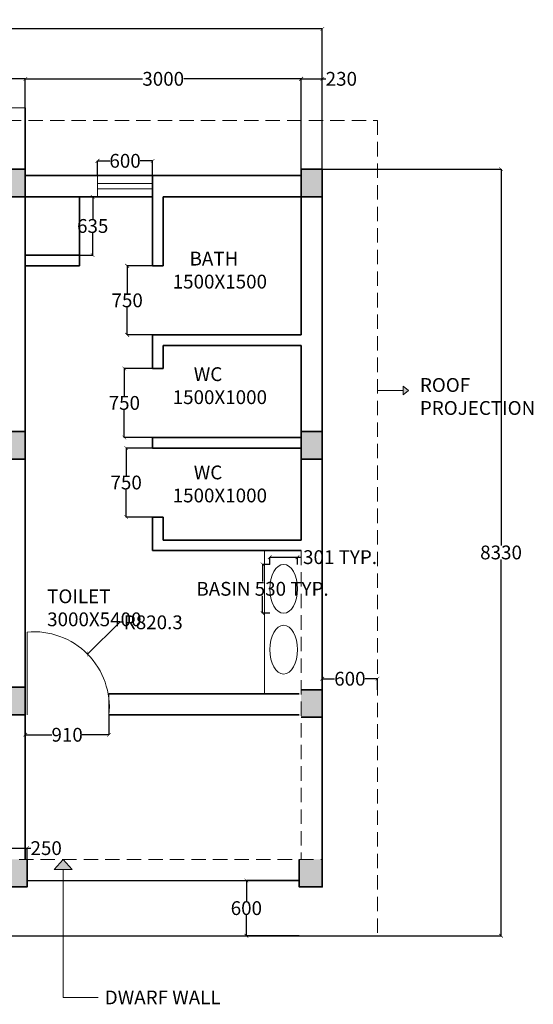
# Model space of a CAD drawing. Units: millimetres. Extents: x 32888 to 53184, y 27889 to 39696.
# Tile 6 of 6: x 47598 to 53184, y 28996 to 39696. Entities that reach past the tile are written whole.
import ezdxf

# ---------------------------------------------------------------- set-up
doc = ezdxf.new("R2010")
doc.units = ezdxf.units.MM
doc.header["$LTSCALE"] = 50
doc.header["$MEASUREMENT"] = 0
doc.linetypes.add('HIDDEN2', pattern=[0.1875, 0.125, -0.0625])
for name, color, linetype, lineweight in [('A-ANNO-DIMS', 2, 'Continuous', 18), ('A-ANNO-SYMB', 7, 'Continuous', 18), ('A-ANNO-SYMB-PATT', 18, 'Continuous', 13), ('A-ANNO-TEXT', 7, 'Continuous', 18), ('A-AREA-IDEN', 7, 'Continuous', 18), ('A-COLS', 1, 'Continuous', 35), ('A-COLS-PATT', 18, 'Continuous', 18), ('A-DOOR', 4, 'Continuous', 18), ('A-FLOR-FIXT', 9, 'Continuous', 18), ('A-GLAZ', 4, 'Continuous', 18), ('A-ROOF-OVHD', 8, 'HIDDEN2', 18), ('A-WALL', 7, 'Continuous', 35), ('A-WALL-HIDN', 7, 'HIDDEN2', 18), ('A-WALL-LOW', 7, 'Continuous', 25)]:
    doc.layers.add(name, color=color, linetype=linetype, lineweight=lineweight)
doc.styles.get("Standard").update_dxf_attribs({"font": 'arial.ttf'})
doc.dimstyles.get("Standard").update_dxf_attribs({"dimtxt": 150, "dimasz": 40, "dimexe": 0.18, "dimexo": 0.0625, "dimgap": 0.09, "dimtad": 0, "dimtih": 1, "dimtoh": 1, "dimdec": 0, "dimzin": 0, "dimdsep": 46, "dimtxsty": 'Standard', "dimblk": 'ARCHTICK', "dimcen": 0, "dimadec": 0, "dimazin": 0, "dimtfac": 1, "dimtdec": 0, "dimtofl": 0, "dimtmove": 0, "dimatfit": 3, "dimldrblk": 'ARCHTICK', "dimfxl": 1, "dimtolj": 1, "dimtzin": 0, "dimarcsym": 1})

# ---------------------------------------------------------------- blocks, each defined once
blk = doc.blocks.new('_ArchTick')
at = {"color": 0, "linetype": 'ByBlock', "const_width": 0.15}
blk.add_lwpolyline([(-0.5, -0.5), (0.5, 0.5)], dxfattribs=at)
blk = doc.blocks.new('*D8')
at = {"layer": 'A-ANNO-DIMS', "color": 0, "lineweight": -2, "ltscale": 50, "transparency": 16777216}
for p, q in [((47429, 30571), (47429, 30693)), ((47429, 30693), (47679, 30693)), ((47679, 30571), (47679, 30693)), ((47679, 30693), (47719, 30693))]:
    blk.add_line(p, q, dxfattribs=at)
at = {"layer": 'Defpoints', "color": 0, "ltscale": 50, "transparency": 16777216}
for p in [(47679, 30693), (47429, 30571), (47679, 30571)]:
    blk.add_point(p, dxfattribs=at)
at = {"layer": 'A-ANNO-DIMS', "color": 0, "lineweight": -2, "ltscale": 50, "transparency": 16777216, "xscale": 40, "yscale": 40, "zscale": 40, "rotation": 180}
blk.add_blockref('_ArchTick', (47429, 30693), dxfattribs=at)
at = {"layer": 'A-ANNO-DIMS', "color": 0, "lineweight": -2, "ltscale": 50, "transparency": 16777216, "xscale": 40, "yscale": 40, "zscale": 40}
blk.add_blockref('_ArchTick', (47679, 30693), dxfattribs=at)
at = {"layer": 'A-ANNO-DIMS', "color": 0, "ltscale": 50, "transparency": 16777216, "insert": (47886, 30693), "char_height": 150, "attachment_point": 5}
blk.add_mtext('\\A1;250', dxfattribs=at)
blk = doc.blocks.new('*D10')
at = {"layer": 'A-ANNO-DIMS', "color": 0, "lineweight": -2, "ltscale": 50, "transparency": 16777216}
for p, q in [((50639, 30341), (50063, 30341)), ((50063, 30341), (50063, 30118)), ((50063, 29741), (50063, 29964)), ((50639, 29741), (50063, 29741))]:
    blk.add_line(p, q, dxfattribs=at)
at = {"layer": 'Defpoints', "color": 0, "ltscale": 50, "transparency": 16777216}
for p in [(50639, 30341), (50063, 29741), (50639, 29741)]:
    blk.add_point(p, dxfattribs=at)
at = {"layer": 'A-ANNO-DIMS', "color": 0, "lineweight": -2, "ltscale": 50, "transparency": 16777216, "xscale": 40, "yscale": 40, "zscale": 40}
for p, rotation in [((50063, 30341), 90), ((50063, 29741), 270)]:
    blk.add_blockref('_ArchTick', p, dxfattribs=dict(at, rotation=rotation))
at = {"layer": 'A-ANNO-DIMS', "color": 0, "ltscale": 50, "transparency": 16777216, "insert": (50063, 30041), "char_height": 150, "attachment_point": 5}
blk.add_mtext('\\A1;600', dxfattribs=at)
blk = doc.blocks.new('*D11')
at = {"layer": 'A-ANNO-DIMS', "color": 0, "lineweight": -2, "ltscale": 50, "transparency": 16777216}
for p, q in [((50889, 32415), (50889, 32534)), ((50889, 32534), (51023, 32534)), ((51489, 32534), (51355, 32534)), ((51489, 32415), (51489, 32534))]:
    blk.add_line(p, q, dxfattribs=at)
at = {"layer": 'Defpoints', "color": 0, "ltscale": 50, "transparency": 16777216}
for p in [(51489, 32534), (50889, 32414), (51489, 32414)]:
    blk.add_point(p, dxfattribs=at)
at = {"layer": 'A-ANNO-DIMS', "color": 0, "lineweight": -2, "ltscale": 50, "transparency": 16777216, "xscale": 40, "yscale": 40, "zscale": 40, "rotation": 180}
blk.add_blockref('_ArchTick', (50889, 32534), dxfattribs=at)
at = {"layer": 'A-ANNO-DIMS', "color": 0, "lineweight": -2, "ltscale": 50, "transparency": 16777216, "xscale": 40, "yscale": 40, "zscale": 40}
blk.add_blockref('_ArchTick', (51489, 32534), dxfattribs=at)
at = {"layer": 'A-ANNO-DIMS', "color": 0, "ltscale": 50, "transparency": 16777216, "insert": (51189, 32534), "char_height": 150, "attachment_point": 5}
blk.add_mtext('\\A1;600', dxfattribs=at)
blk = doc.blocks.new('*D27')
at = {"layer": 'A-ANNO-DIMS', "color": 0, "lineweight": -2, "ltscale": 50, "transparency": 16777216}
for p, q in [((49044, 35041), (48756, 35041)), ((48756, 35041), (48756, 34743)), ((48756, 34291), (48756, 34589)), ((49044, 34291), (48756, 34291))]:
    blk.add_line(p, q, dxfattribs=at)
at = {"layer": 'Defpoints', "color": 0, "ltscale": 50, "transparency": 16777216}
for p in [(49044, 35041), (48756, 34291), (49044, 34291)]:
    blk.add_point(p, dxfattribs=at)
at = {"layer": 'A-ANNO-DIMS', "color": 0, "lineweight": -2, "ltscale": 50, "transparency": 16777216, "xscale": 40, "yscale": 40, "zscale": 40}
for p, rotation in [((48756, 35041), 90), ((48756, 34291), 270)]:
    blk.add_blockref('_ArchTick', p, dxfattribs=dict(at, rotation=rotation))
at = {"layer": 'A-ANNO-DIMS', "color": 0, "ltscale": 50, "transparency": 16777216, "insert": (48756, 34666), "char_height": 150, "attachment_point": 5}
blk.add_mtext('\\A1;750', dxfattribs=at)
blk = doc.blocks.new('*D28')
at = {"layer": 'A-ANNO-DIMS', "color": 0, "lineweight": -2, "ltscale": 50, "transparency": 16777216}
for p, q in [((49044, 35906), (48736, 35906)), ((48736, 35906), (48736, 35608)), ((48736, 35156), (48736, 35454)), ((49044, 35156), (48736, 35156))]:
    blk.add_line(p, q, dxfattribs=at)
at = {"layer": 'Defpoints', "color": 0, "ltscale": 50, "transparency": 16777216}
for p in [(49044, 35906), (48736, 35156), (49044, 35156)]:
    blk.add_point(p, dxfattribs=at)
at = {"layer": 'A-ANNO-DIMS', "color": 0, "lineweight": -2, "ltscale": 50, "transparency": 16777216, "xscale": 40, "yscale": 40, "zscale": 40}
for p, rotation in [((48736, 35906), 90), ((48736, 35156), 270)]:
    blk.add_blockref('_ArchTick', p, dxfattribs=dict(at, rotation=rotation))
at = {"layer": 'A-ANNO-DIMS', "color": 0, "ltscale": 50, "transparency": 16777216, "insert": (48736, 35531), "char_height": 150, "attachment_point": 5}
blk.add_mtext('\\A1;750', dxfattribs=at)
blk = doc.blocks.new('*D29')
at = {"layer": 'A-ANNO-DIMS', "color": 0, "lineweight": -2, "ltscale": 50, "transparency": 16777216}
for p, q in [((49044, 37021), (48767, 37021)), ((48767, 37021), (48767, 36723)), ((48767, 36271), (48767, 36569)), ((49044, 36271), (48767, 36271))]:
    blk.add_line(p, q, dxfattribs=at)
at = {"layer": 'Defpoints', "color": 0, "ltscale": 50, "transparency": 16777216}
for p in [(48767, 37021), (49044, 37021), (49044, 36271)]:
    blk.add_point(p, dxfattribs=at)
at = {"layer": 'A-ANNO-DIMS', "color": 0, "lineweight": -2, "ltscale": 50, "transparency": 16777216, "xscale": 40, "yscale": 40, "zscale": 40}
for p, rotation in [((48767, 37021), 90), ((48767, 36271), 270)]:
    blk.add_blockref('_ArchTick', p, dxfattribs=dict(at, rotation=rotation))
at = {"layer": 'A-ANNO-DIMS', "color": 0, "ltscale": 50, "transparency": 16777216, "insert": (48767, 36646), "char_height": 150, "attachment_point": 5}
blk.add_mtext('\\A1;750', dxfattribs=at)
blk = doc.blocks.new('*D30')
at = {"layer": 'A-ANNO-DIMS', "color": 0, "lineweight": -2, "ltscale": 50, "transparency": 16777216}
for p, q in [((48249, 37771), (48392, 37771)), ((48392, 37771), (48392, 37530)), ((48392, 37136), (48392, 37377)), ((48249, 37136), (48392, 37136))]:
    blk.add_line(p, q, dxfattribs=at)
at = {"layer": 'Defpoints', "color": 0, "ltscale": 50, "transparency": 16777216}
for p in [(48249, 37771), (48392, 37771), (48249, 37136)]:
    blk.add_point(p, dxfattribs=at)
at = {"layer": 'A-ANNO-DIMS', "color": 0, "lineweight": -2, "ltscale": 50, "transparency": 16777216, "xscale": 40, "yscale": 40, "zscale": 40}
for p, rotation in [((48392, 37771), 90), ((48392, 37136), 270)]:
    blk.add_blockref('_ArchTick', p, dxfattribs=dict(at, rotation=rotation))
at = {"layer": 'A-ANNO-DIMS', "color": 0, "ltscale": 50, "transparency": 16777216, "insert": (48392, 37454), "char_height": 150, "attachment_point": 5}
blk.add_mtext('\\A1;635', dxfattribs=at)
blk = doc.blocks.new('*D31')
at = {"layer": 'A-ANNO-DIMS', "color": 0, "lineweight": -2, "ltscale": 50, "transparency": 16777216}
for p, q in [((48444, 38001), (48444, 38162)), ((48444, 38162), (48578, 38162)), ((49044, 38162), (48910, 38162)), ((49044, 38001), (49044, 38162))]:
    blk.add_line(p, q, dxfattribs=at)
at = {"layer": 'Defpoints', "color": 0, "ltscale": 50, "transparency": 16777216}
for p in [(49044, 38162), (48444, 38001), (49044, 38001)]:
    blk.add_point(p, dxfattribs=at)
at = {"layer": 'A-ANNO-DIMS', "color": 0, "lineweight": -2, "ltscale": 50, "transparency": 16777216, "xscale": 40, "yscale": 40, "zscale": 40, "rotation": 180}
blk.add_blockref('_ArchTick', (48444, 38162), dxfattribs=at)
at = {"layer": 'A-ANNO-DIMS', "color": 0, "lineweight": -2, "ltscale": 50, "transparency": 16777216, "xscale": 40, "yscale": 40, "zscale": 40}
blk.add_blockref('_ArchTick', (49044, 38162), dxfattribs=at)
at = {"layer": 'A-ANNO-DIMS', "color": 0, "ltscale": 50, "transparency": 16777216, "insert": (48744, 38162), "char_height": 150, "attachment_point": 5}
blk.add_mtext('\\A1;600', dxfattribs=at)
blk = doc.blocks.new('*D48')
at = {"layer": 'A-ANNO-DIMS', "color": 0, "lineweight": -2, "ltscale": 50, "transparency": 16777216}
for p, q in [((50659, 38071), (50659, 39053)), ((50659, 39053), (50889, 39053)), ((50889, 38071), (50889, 39053)), ((50889, 39053), (50929, 39053))]:
    blk.add_line(p, q, dxfattribs=at)
at = {"layer": 'Defpoints', "color": 0, "ltscale": 50, "transparency": 16777216}
for p in [(50889, 39053), (50659, 38071), (50889, 38071)]:
    blk.add_point(p, dxfattribs=at)
at = {"layer": 'A-ANNO-DIMS', "color": 0, "lineweight": -2, "ltscale": 50, "transparency": 16777216, "xscale": 40, "yscale": 40, "zscale": 40, "rotation": 180}
blk.add_blockref('_ArchTick', (50659, 39053), dxfattribs=at)
at = {"layer": 'A-ANNO-DIMS', "color": 0, "lineweight": -2, "ltscale": 50, "transparency": 16777216, "xscale": 40, "yscale": 40, "zscale": 40}
blk.add_blockref('_ArchTick', (50889, 39053), dxfattribs=at)
at = {"layer": 'A-ANNO-DIMS', "color": 0, "ltscale": 50, "transparency": 16777216, "insert": (51096, 39053), "char_height": 150, "attachment_point": 5}
blk.add_mtext('\\A1;230', dxfattribs=at)
blk = doc.blocks.new('*D49')
at = {"layer": 'A-ANNO-DIMS', "color": 0, "lineweight": -2, "ltscale": 50, "transparency": 16777216}
for p, q in [((47659, 38001), (47659, 39053)), ((47659, 39053), (48935, 39053)), ((50659, 39053), (49383, 39053)), ((50659, 38001), (50659, 39053))]:
    blk.add_line(p, q, dxfattribs=at)
at = {"layer": 'Defpoints', "color": 0, "ltscale": 50, "transparency": 16777216}
for p in [(47659, 39053), (47659, 38001), (50659, 38001)]:
    blk.add_point(p, dxfattribs=at)
at = {"layer": 'A-ANNO-DIMS', "color": 0, "lineweight": -2, "ltscale": 50, "transparency": 16777216, "xscale": 40, "yscale": 40, "zscale": 40, "rotation": 180}
blk.add_blockref('_ArchTick', (47659, 39053), dxfattribs=at)
at = {"layer": 'A-ANNO-DIMS', "color": 0, "lineweight": -2, "ltscale": 50, "transparency": 16777216, "xscale": 40, "yscale": 40, "zscale": 40}
blk.add_blockref('_ArchTick', (50659, 39053), dxfattribs=at)
at = {"layer": 'A-ANNO-DIMS', "color": 0, "ltscale": 50, "transparency": 16777216, "insert": (49159, 39053), "char_height": 150, "attachment_point": 5}
blk.add_mtext('\\A1;3000', dxfattribs=at)
blk = doc.blocks.new('*D50')
at = {"layer": 'A-ANNO-DIMS', "color": 0, "lineweight": -2, "ltscale": 50, "transparency": 16777216}
for p, q in [((47429, 39053), (47389, 39053)), ((47429, 38071), (47429, 39053)), ((47659, 39053), (47429, 39053)), ((47659, 38071), (47659, 39053))]:
    blk.add_line(p, q, dxfattribs=at)
at = {"layer": 'Defpoints', "color": 0, "ltscale": 50, "transparency": 16777216}
for p in [(47429, 39053), (47429, 38071), (47659, 38071)]:
    blk.add_point(p, dxfattribs=at)
at = {"layer": 'A-ANNO-DIMS', "color": 0, "lineweight": -2, "ltscale": 50, "transparency": 16777216, "xscale": 40, "yscale": 40, "zscale": 40}
for p, rotation in [((47429, 39053), 179.9999999999982), ((47659, 39053), 359.9999999999982)]:
    blk.add_blockref('_ArchTick', p, dxfattribs=dict(at, rotation=rotation))
at = {"layer": 'A-ANNO-DIMS', "color": 0, "ltscale": 50, "transparency": 16777216, "insert": (47222, 39053), "char_height": 150, "attachment_point": 5}
blk.add_mtext('\\A1;230', dxfattribs=at)
blk = doc.blocks.new('*D56')
at = {"layer": 'A-ANNO-DIMS', "color": 0, "lineweight": -2, "ltscale": 50, "transparency": 16777216}
for p, q in [((47659, 32141), (47659, 31925)), ((48569, 32141), (48569, 31925)), ((47659, 31925), (47948, 31925)), ((48569, 31925), (48279, 31925))]:
    blk.add_line(p, q, dxfattribs=at)
at = {"layer": 'Defpoints', "color": 0, "ltscale": 50, "transparency": 16777216}
for p in [(47659, 32141), (48569, 32141), (47659, 31925)]:
    blk.add_point(p, dxfattribs=at)
at = {"layer": 'A-ANNO-DIMS', "color": 0, "lineweight": -2, "ltscale": 50, "transparency": 16777216, "xscale": 40, "yscale": 40, "zscale": 40, "rotation": 180}
blk.add_blockref('_ArchTick', (47659, 31925), dxfattribs=at)
at = {"layer": 'A-ANNO-DIMS', "color": 0, "lineweight": -2, "ltscale": 50, "transparency": 16777216, "xscale": 40, "yscale": 40, "zscale": 40}
blk.add_blockref('_ArchTick', (48569, 31925), dxfattribs=at)
at = {"layer": 'A-ANNO-DIMS', "color": 0, "ltscale": 50, "transparency": 16777216, "insert": (48114, 31925), "char_height": 150, "attachment_point": 5}
blk.add_mtext('\\A1;910', dxfattribs=at)
blk = doc.blocks.new('*D57')
at = {"layer": 'A-ANNO-DIMS', "color": 0, "lineweight": -2, "ltscale": 50, "transparency": 16777216}
for p, q in [((35169, 38001), (35169, 39597)), ((35169, 39597), (42754, 39597)), ((50889, 39597), (43304, 39597)), ((50889, 38001), (50889, 39597))]:
    blk.add_line(p, q, dxfattribs=at)
at = {"layer": 'Defpoints', "color": 0, "ltscale": 50, "transparency": 16777216}
for p in [(50889, 39597), (35169, 38001), (50889, 38001)]:
    blk.add_point(p, dxfattribs=at)
at = {"layer": 'A-ANNO-DIMS', "color": 0, "lineweight": -2, "ltscale": 50, "transparency": 16777216, "xscale": 40, "yscale": 40, "zscale": 40, "rotation": 180}
blk.add_blockref('_ArchTick', (35169, 39597), dxfattribs=at)
at = {"layer": 'A-ANNO-DIMS', "color": 0, "lineweight": -2, "ltscale": 50, "transparency": 16777216, "xscale": 40, "yscale": 40, "zscale": 40}
blk.add_blockref('_ArchTick', (50889, 39597), dxfattribs=at)
at = {"layer": 'A-ANNO-DIMS', "color": 0, "ltscale": 50, "transparency": 16777216, "insert": (43029, 39597), "char_height": 150, "attachment_point": 5}
blk.add_mtext('\\A1;15720', dxfattribs=at)
blk = doc.blocks.new('SANITARY-OVAL')
blk.add_ellipse((0, 0), major_axis=(0, -265), ratio=0.567568)
blk = doc.blocks.new('COLUMN-IN-WALL-230x300')
for points in [[(0, 300), (230, 300)], [(230, 0), (0, 0)]]:
    blk.add_lwpolyline(points)
blk = doc.blocks.new('*D75')
at = {"layer": 'A-ANNO-DIMS', "color": 0, "lineweight": -2, "ltscale": 50, "transparency": 16777216}
for p, q in [((50318, 33776), (50238, 33776)), ((50239, 33776), (50239, 33589)), ((50239, 33246), (50239, 33433)), ((50318, 33246), (50238, 33246))]:
    blk.add_line(p, q, dxfattribs=at)
at = {"layer": 'Defpoints', "color": 0, "ltscale": 50, "transparency": 16777216}
for p in [(50239, 33776), (50318, 33776), (50318, 33246)]:
    blk.add_point(p, dxfattribs=at)
at = {"layer": 'A-ANNO-DIMS', "color": 0, "lineweight": -2, "ltscale": 50, "transparency": 16777216, "xscale": 40, "yscale": 40, "zscale": 40}
for p, rotation in [((50239, 33776), 90), ((50239, 33246), 270)]:
    blk.add_blockref('_ArchTick', p, dxfattribs=dict(at, rotation=rotation))
at = {"layer": 'A-ANNO-DIMS', "color": 0, "ltscale": 50, "transparency": 16777216, "insert": (50239, 33511), "char_height": 150, "attachment_point": 5}
blk.add_mtext('\\A1;BASIN 530 TYP.', dxfattribs=at)
blk = doc.blocks.new('*D76')
at = {"layer": 'A-ANNO-DIMS', "color": 0, "lineweight": -2, "ltscale": 50, "transparency": 16777216}
for p, q in [((50318, 33776), (50318, 33856)), ((50318, 33855), (50619, 33855)), ((50619, 33776), (50619, 33856)), ((50619, 33855), (50659, 33855))]:
    blk.add_line(p, q, dxfattribs=at)
at = {"layer": 'Defpoints', "color": 0, "ltscale": 50, "transparency": 16777216}
for p in [(50619, 33855), (50318, 33776), (50619, 33776)]:
    blk.add_point(p, dxfattribs=at)
at = {"layer": 'A-ANNO-DIMS', "color": 0, "lineweight": -2, "ltscale": 50, "transparency": 16777216, "xscale": 40, "yscale": 40, "zscale": 40, "rotation": 180}
blk.add_blockref('_ArchTick', (50318, 33855), dxfattribs=at)
at = {"layer": 'A-ANNO-DIMS', "color": 0, "lineweight": -2, "ltscale": 50, "transparency": 16777216, "xscale": 40, "yscale": 40, "zscale": 40}
blk.add_blockref('_ArchTick', (50619, 33855), dxfattribs=at)
at = {"layer": 'A-ANNO-DIMS', "color": 0, "ltscale": 50, "transparency": 16777216, "insert": (51082, 33855), "char_height": 150, "attachment_point": 5}
blk.add_mtext('\\A1;301 TYP.', dxfattribs=at)
blk = doc.blocks.new('*D77')
at = {"layer": 'A-ANNO-DIMS', "color": 0, "lineweight": -2, "ltscale": 50, "transparency": 16777216}
for p, q in [((50889, 38071), (52833, 38071)), ((52833, 38071), (52833, 33983)), ((52833, 29741), (52833, 33829)), ((43354, 29741), (52833, 29741))]:
    blk.add_line(p, q, dxfattribs=at)
at = {"layer": 'Defpoints', "color": 0, "ltscale": 50, "transparency": 16777216}
for p in [(50889, 38071), (43354, 29741), (52833, 29741)]:
    blk.add_point(p, dxfattribs=at)
at = {"layer": 'A-ANNO-DIMS', "color": 0, "lineweight": -2, "ltscale": 50, "transparency": 16777216, "xscale": 40, "yscale": 40, "zscale": 40}
for p, rotation in [((52833, 38071), 90), ((52833, 29741), 270)]:
    blk.add_blockref('_ArchTick', p, dxfattribs=dict(at, rotation=rotation))
at = {"layer": 'A-ANNO-DIMS', "color": 0, "ltscale": 50, "transparency": 16777216, "insert": (52833, 33906), "char_height": 150, "attachment_point": 5}
blk.add_mtext('\\A1;8330', dxfattribs=at)
blk = doc.blocks.new('*D79')
at = {"layer": 'A-ANNO-DIMS', "color": 0, "lineweight": -2, "ltscale": 50, "transparency": 16777216}
for p, q in [((48686, 33147), (48336, 32801)), ((48726, 33147), (48686, 33147))]:
    blk.add_line(p, q, dxfattribs=at)
at = {"layer": 'Defpoints', "color": 0, "ltscale": 50, "transparency": 16777216}
for p in [(48336, 32801), (47753, 32224)]:
    blk.add_point(p, dxfattribs=at)
at = {"layer": 'A-ANNO-DIMS', "color": 0, "lineweight": -2, "ltscale": 50, "transparency": 16777216, "xscale": 40, "yscale": 40, "zscale": 40, "rotation": 224.6799242760047}
blk.add_blockref('_ArchTick', (48336, 32801), dxfattribs=at)
at = {"layer": 'A-ANNO-DIMS', "color": 0, "ltscale": 50, "transparency": 16777216, "insert": (49051, 33147), "char_height": 150, "attachment_point": 5}
blk.add_mtext('\\A1;R820.3', dxfattribs=at)

msp = doc.modelspace()

# ---------------------------------------------------------------- hatches: boundary and pattern name
at = {"layer": 'A-ANNO-SYMB-PATT', "ltscale": 50}
h = msp.add_hatch(color=256, dxfattribs=at)
h.dxf.hatch_style = 1
h.paths.add_polyline_path([(36870.29, 30540.94), (36772.99, 30430.6), (36870.29, 30430.6), (36967.6, 30430.6)])
h.paths.add_polyline_path([(48072.03, 30571.01), (47974.72, 30460.67), (48072.03, 30460.67), (48169.34, 30460.67)])
h.paths.add_polyline_path([(51769.69, 35712.9), (51769.69, 35665.99), (51769.69, 35619.08), (51826.03, 35665.99)])
at = {"layer": 'A-COLS-PATT', "ltscale": 50}
h = msp.add_hatch(color=256, dxfattribs=at)
h.dxf.hatch_style = 1
h.paths.add_polyline_path([(35398.95, 38071.01), (35168.95, 38071.01), (35168.95, 37771.01), (35398.95, 37771.01)])
h.paths.add_polyline_path([(39628.95, 38071.01), (39398.95, 38071.01), (39398.95, 37771.01), (39628.95, 37771.01)])
h.paths.add_polyline_path([(43903.95, 38071.01), (43673.95, 38071.01), (43673.95, 37771.01), (43903.95, 37771.01)])
h.paths.add_polyline_path([(47658.95, 38071.01), (47428.95, 38071.01), (47428.95, 37771.01), (47658.95, 37771.01)])
h.paths.add_polyline_path([(50888.95, 38071.01), (50658.95, 38071.01), (50658.95, 37771.01), (50888.95, 37771.01)])
h.paths.add_polyline_path([(50888.95, 35221.01), (50658.95, 35221.01), (50658.95, 34921.01), (50888.95, 34921.01)])
h.paths.add_polyline_path([(47658.95, 35221.01), (47428.95, 35221.01), (47428.95, 34921.01), (47658.95, 34921.01)])
h.paths.add_polyline_path([(39628.95, 35071.01), (39628.95, 35221.01), (39398.95, 35221.01), (39398.95, 34921.01), (39628.95, 34921.01)])
h.paths.add_polyline_path([(35398.95, 35221.01), (35168.95, 35221.01), (35168.95, 34921.01), (35398.95, 34921.01)])
h.paths.add_polyline_path([(35398.95, 32371.01), (35168.95, 32371.01), (35168.95, 32071.01), (35398.95, 32071.01)])
h.paths.add_polyline_path([(35418.95, 30571.01), (35168.95, 30571.01), (35168.95, 30271.01), (35418.95, 30271.01)])
h.paths.add_polyline_path([(39642.61, 30571.01), (39392.61, 30571.01), (39392.61, 30271.01), (39642.61, 30271.01)])
h.paths.add_polyline_path([(39628.95, 32371.01), (39398.95, 32371.01), (39398.95, 32071.01), (39628.95, 32071.01)])
h.paths.add_polyline_path([(43903.95, 32371.01), (43673.95, 32371.01), (43673.95, 32071.01), (43903.95, 32071.01)])
h.paths.add_polyline_path([(43903.95, 30571.01), (43653.95, 30571.01), (43653.95, 30271.01), (43903.95, 30271.01)])
h.paths.add_polyline_path([(47658.95, 32441.01), (47428.95, 32441.01), (47428.95, 32141.01), (47658.95, 32141.01)])
h.paths.add_polyline_path([(50888.95, 32414.45), (50658.95, 32414.45), (50658.95, 32114.45), (50888.95, 32114.45)])
h.paths.add_polyline_path([(50888.95, 30571.01), (50638.95, 30571.01), (50638.95, 30271.01), (50888.95, 30271.01)])
h.paths.add_polyline_path([(47678.95, 30571.01), (47428.95, 30571.01), (47428.95, 30341.01), (47678.95, 30341.01)])
h.paths.add_polyline_path([(47678.95, 30341.01), (47428.95, 30341.01), (47428.95, 30271.01), (47678.95, 30271.01)])

# ---------------------------------------------------------------- linework, layer by layer
at = {"layer": 'A-ANNO-SYMB', "ltscale": 50}
for p, q in [((51488.95, 35665.99), (51769.69, 35665.99)), ((51826.03, 35665.99), (51769.69, 35712.9)), ((51769.69, 35712.9), (51769.69, 35665.99)), ((51826.03, 35665.99), (51769.69, 35619.08)), ((51769.69, 35619.08), (51769.69, 35665.99)), ((48072.03, 30571.01), (47974.72, 30460.67)), ((48072.03, 30571.01), (48169.34, 30460.67)), ((47974.72, 30460.67), (48072.03, 30460.67)), ((48072.03, 29069.54), (48072.03, 30460.67)), ((48169.34, 30460.67), (48072.03, 30460.67)), ((48453.08, 29069.54), (48072.03, 29069.54))]:
    msp.add_line(p, q, dxfattribs=at)
at = {"layer": 'A-COLS'}
for points in [[(47658.95, 38071.01), (47428.95, 38071.01)], [(50888.95, 38071.01), (50658.95, 38071.01)], [(47658.95, 32441.01), (47428.95, 32441.01)], [(50888.95, 32414.45), (50658.95, 32414.45)], [(50888.95, 32114.45), (50658.95, 32114.45)], [(47428.95, 30271.01), (47678.95, 30271.01), (47678.95, 30571.01)]]:
    msp.add_lwpolyline(points, dxfattribs=at)
at = {"layer": 'A-DOOR', "ltscale": 50}
for p, q in [((47658.95, 32141.01), (47658.95, 33041.01)), ((47678.95, 32141.01), (47678.95, 33041.01)), ((47658.95, 32371.01), (47658.95, 32141.01)), ((48568.95, 32371.01), (48568.95, 32141.01))]:
    msp.add_line(p, q, dxfattribs=at)
msp.add_arc((47752.82, 32224), 820.34, 354.193493, 95.166338, dxfattribs=at)
at = {"layer": 'A-FLOR-FIXT'}
msp.add_line((50258.95, 33926.01), (50258.95, 32371.01), dxfattribs=at)
at = {"layer": 'A-GLAZ'}
for p, q in [((48443.95, 37771.01), (48443.95, 38001.01)), ((48443.95, 37916.01), (49043.95, 37916.01)), ((48443.95, 37856.01), (49043.95, 37856.01))]:
    msp.add_line(p, q, dxfattribs=at)
at = {"layer": 'A-ROOF-OVHD', "ltscale": 25}
for p, q in [((34568.95, 38601.01), (51488.95, 38601.01)), ((51488.95, 38601.01), (51488.95, 29741.01)), ((34568.95, 29741.01), (51488.95, 29741.01))]:
    msp.add_line(p, q, dxfattribs=at)
msp.add_lwpolyline([(47658.95, 38736.01), (46298.95, 38736.01)], dxfattribs=at)
at = {"layer": 'A-WALL'}
for p, q in [((47658.95, 38736.01), (47658.95, 30571.01)), ((47658.95, 38001.01), (50658.95, 38001.01)), ((49043.95, 37021.01), (49043.95, 38001.01)), ((50658.95, 38071.01), (50658.95, 36271.01)), ((46413.95, 37771.01), (49043.95, 37771.01)), ((48248.6, 37021.01), (48248.6, 37771.01)), ((49158.95, 37771.01), (50888.95, 37771.01)), ((49158.95, 37021.01), (49158.95, 37771.01)), ((47658.95, 37136.01), (48248.6, 37136.01)), ((47658.95, 37021.01), (48248.6, 37021.01)), ((49158.95, 37021.01), (49043.95, 37021.01)), ((50658.95, 36271.01), (49043.95, 36271.01)), ((49043.95, 35906.01), (49043.95, 36271.01)), ((50658.95, 36156.01), (49158.95, 36156.01)), ((49158.95, 35906.01), (49158.95, 36156.01)), ((50658.95, 36156.01), (50658.95, 34041.01)), ((49158.95, 35906.01), (49043.95, 35906.01)), ((50658.95, 35156.01), (49043.95, 35156.01)), ((49043.95, 35041.01), (49043.95, 35156.01)), ((50658.95, 35041.01), (49043.95, 35041.01)), ((49043.95, 33926.01), (49043.95, 34291.01)), ((49158.95, 34291.01), (49043.95, 34291.01)), ((49158.95, 34041.01), (49158.95, 34291.01)), ((50658.95, 34041.01), (49158.95, 34041.01)), ((50658.95, 33926.01), (49043.95, 33926.01)), ((48568.95, 32371.01), (50638.95, 32371.01)), ((43903.95, 32141.01), (47658.95, 32141.01)), ((48568.95, 32141.01), (50638.95, 32141.01))]:
    msp.add_line(p, q, dxfattribs=at)
msp.add_lwpolyline([(50638.95, 30571.01), (50638.95, 30271.01), (50888.95, 30271.01), (50888.95, 38071.01)], dxfattribs=at)
at = {"layer": 'A-WALL-HIDN', "ltscale": 25}
for p, q in [((50658.95, 33926.01), (50658.95, 30571.01)), ((35168.95, 30571.01), (50888.95, 30571.01))]:
    msp.add_line(p, q, dxfattribs=at)
at = {"layer": 'A-WALL-LOW'}
msp.add_line((47678.95, 30341.01), (50638.95, 30341.01), dxfattribs=at)

# ---------------------------------------------------------------- block references
at = {"layer": 'A-COLS'}
for p in [(47428.95, 34921.01), (50658.95, 34921.01)]:
    msp.add_blockref('COLUMN-IN-WALL-230x300', p, dxfattribs=at)
at = {"layer": 'A-FLOR-FIXT'}
for p in [(50468.62, 33510.84), (50468.62, 32850.02)]:
    msp.add_blockref('SANITARY-OVAL', p, dxfattribs=at)

# ---------------------------------------------------------------- texts
at = {"layer": 'A-ANNO-TEXT', "ltscale": 50, "char_height": 150, "attachment_point": 1}
for s, insert in [('ROOF\\PPROJECTION', (51950.37, 35801.05)), ('DWARF WALL', (48523.07, 29145.84))]:
    msp.add_mtext_dynamic_manual_height_columns(s, width=2240.7113, gutter_width=1, heights=[0], dxfattribs=dict(at, insert=insert))
at = {"layer": 'A-AREA-IDEN', "ltscale": 50, "char_height": 150, "attachment_point": 1}
for s, insert in [('    BATH\\P1500X1500', (49261.88, 37174.3)), ('     WC\\P1500X1000', (49261.88, 35918.53)), ('     WC\\P1500X1000', (49261.88, 34850.59)), ('TOILET\\P3000X5400', (47896.61, 33504.49))]:
    msp.add_mtext_dynamic_manual_height_columns(s, width=901.3249, gutter_width=1, heights=[0], dxfattribs=dict(at, insert=insert))

# ---------------------------------------------------------------- dimensions: what is measured, and where the dimension line sits
at = {"layer": 'A-ANNO-DIMS', "ltscale": 50}
for p1, p2, distance, picture, middle in [((35168.95, 38001.01), (50888.95, 38001.01), 1596.15, '*D57', (43028.95, 39597.16)), ((47658.95, 38071.01), (47428.95, 38071.01), -981.9, '*D50', (47222.13, 39052.91)), ((50658.95, 38001.01), (47658.95, 38001.01), -1051.9, '*D49', (49158.95, 39052.91)), ((50658.95, 38071.01), (50888.95, 38071.01), 981.9, '*D48', (51095.77, 39052.91)), ((48443.95, 38001.01), (49043.95, 38001.01), 160.63, '*D31', (48743.95, 38161.64)), ((48248.6, 37136.01), (48248.6, 37771.01), -143.7, '*D30', (48392.29, 37453.51)), ((49043.95, 36271.01), (49043.95, 37021.01), 276.9, '*D29', (48767.05, 36646.01)), ((49043.95, 35906.01), (49043.95, 35156.01), -308.18, '*D28', (48735.77, 35531.01)), ((49043.95, 35041.01), (49043.95, 34291.01), -288.18, '*D27', (48755.77, 34666.01)), ((50888.95, 32414.45), (51488.95, 32414.45), 119.24, '*D11', (51188.95, 32533.69)), ((48568.95, 32141.01), (47658.95, 32141.01), 215.73, '*D56', (48113.95, 31925.28)), ((47428.95, 30571.01), (47678.95, 30571.01), 121.77, '*D8', (47885.77, 30692.78)), ((50638.95, 30341.01), (50638.95, 29741.01), -575.99, '*D10', (50062.96, 30041.01))]:
    dim = msp.add_aligned_dim(p1=p1, p2=p2, distance=distance, dimstyle='Standard', override={"dimclrd": 0, "dimclre": 0, "dimclrt": 0}, dxfattribs=at)
    dim.commit()
    dim.dimension.update_dxf_attribs({"geometry": picture, "text_midpoint": middle})
dim = msp.add_linear_dim(base=(52833.03, 29741.01), p1=(50888.95, 38071.01), p2=(43353.95, 29741.01), angle=90, dimstyle='Standard', override={"dimdec": 0, "dimlfac": 1, "dimrnd": 0, "dimzin": 0, "dimdsep": 46, "dimlunit": 2}, dxfattribs=at)
dim.commit()
dim.dimension.update_dxf_attribs({"geometry": '*D77', "text_midpoint": (52833.03, 33906.01)})
dim = msp.add_linear_dim(base=(50619.07, 33855.45), p1=(50318.16, 33775.93), p2=(50619.07, 33775.93), text='<> TYP.', dimstyle='Standard', override={"dimdec": 0, "dimlfac": 1, "dimrnd": 0, "dimzin": 0, "dimdsep": 46, "dimlunit": 2}, dxfattribs=at)
dim.commit()
dim.dimension.update_dxf_attribs({"geometry": '*D76', "text_midpoint": (51082.46, 33855.45)})
dim = msp.add_linear_dim(base=(50238.63, 33775.93), p1=(50318.16, 33245.75), p2=(50318.16, 33775.93), angle=90, text='BASIN <> TYP.', dimstyle='Standard', override={"dimdec": 0, "dimlfac": 1, "dimrnd": 0, "dimzin": 0, "dimdsep": 46, "dimlunit": 2}, dxfattribs=at)
dim.commit()
dim.dimension.update_dxf_attribs({"geometry": '*D75', "text_midpoint": (50238.63, 33510.84)})
dim = msp.add_radius_dim(center=(47752.82, 32224), mpoint=(48336.12, 32800.82), dimstyle='Standard', override={"dimdec": 1, "dimlfac": 1, "dimrnd": 0, "dimzin": 0, "dimdsep": 46, "dimlunit": 2}, dxfattribs=at)
dim.commit()
dim.dimension.update_dxf_attribs({"geometry": '*D79', "text_midpoint": (49051.05, 33146.91), "dimtype": 164})

doc.saveas('drawing.dxf')
